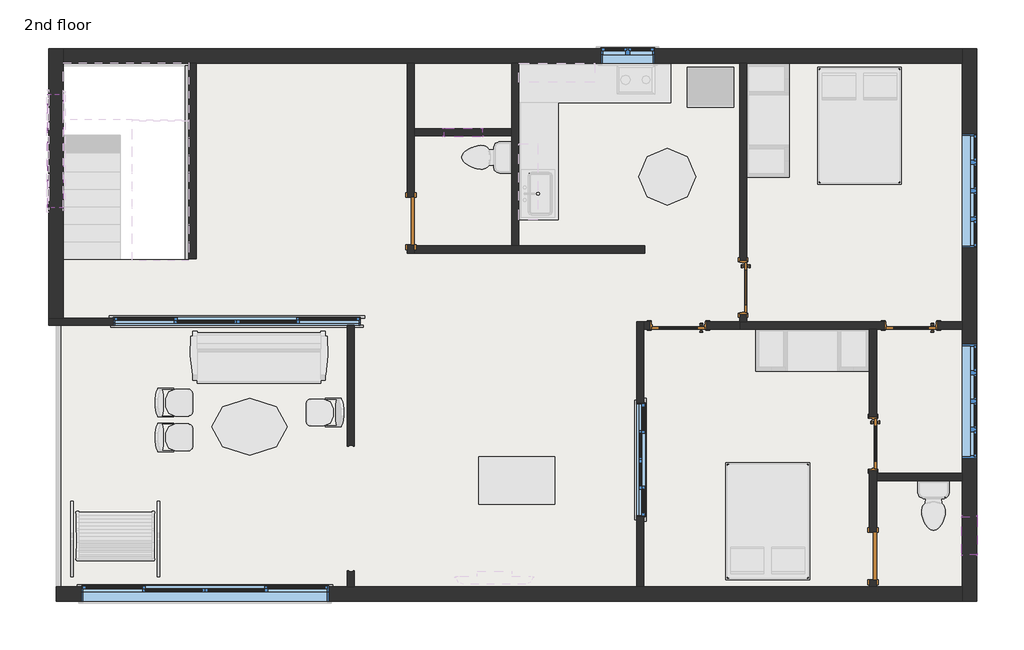
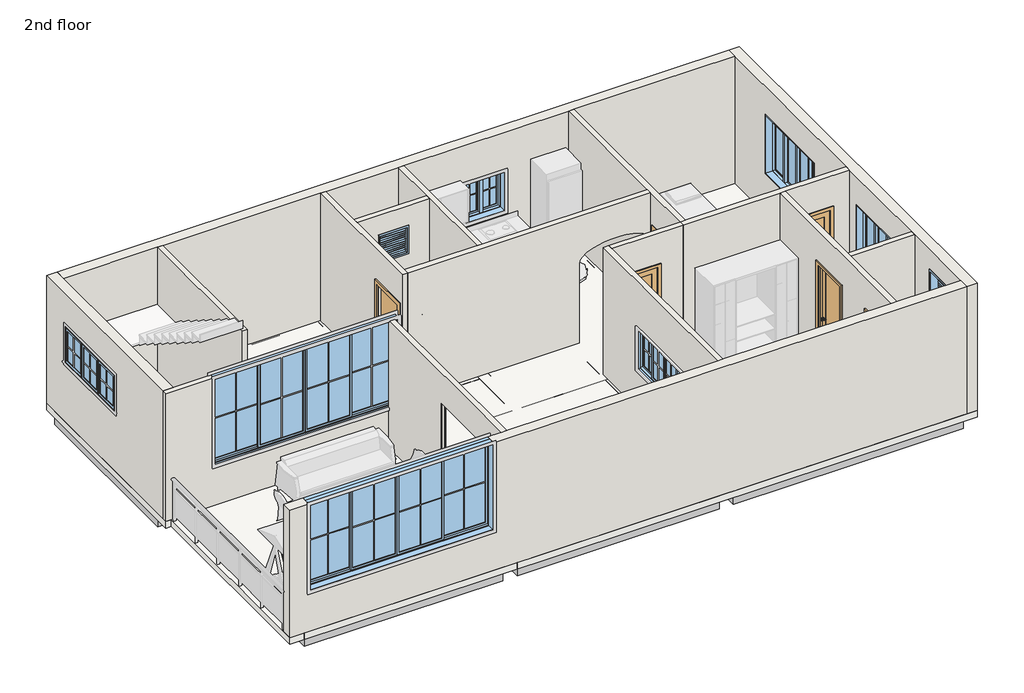
# One storey, part 1 of 2: 17 walls, 9 beams, 9 windows, 6 doors, 1 slab.
"""IFC4 building model written with IfcOpenShell, lengths in millimetres."""

from ifc_helpers import new_model, si_unit, point, frame, origin, place, context, project, spatial, polyline, ellipse_curve, trimmed, outline, extrude, faceted_brep, transform, mapped, element, save
from ifc_brep_helpers import plane_surface, extruded_surface, advanced_brep
from components import door_643e272e, door_51292941, door_214872d5, window_33d4544c, window_339605e1, window_5487fb6d, window_d39e7ecb, window_f2d8fef0, window_cbca41e3, window_8ea0b4a1, window_cd2bb1e7

model = new_model("IFC4")

# Units and contexts
model_context = context("Model", 3, world=origin())
ifc_project = project(units=[si_unit("LENGTHUNIT", "METRE", prefix="MILLI")], contexts=[model_context])

# Site, building, storey
site = spatial("IfcSite", under=ifc_project)
building = spatial("IfcBuilding", under=site)
storey = spatial("IfcBuildingStorey", under=building, Name="2nd floor", Elevation=7010.4)

# Beams
placement = place(None, origin())
element("IfcBeam", 1, ObjectType="Concrete-Rectangular Beam", at=placement, inside=storey, context=model_context, shape_type="Brep", body=[
    faceted_brep([(-12452.868339, 913.093496, 7010.4), (-12452.868339, 684.493496, 7010.4), (-8179.318339, 684.493496, 7010.4), (-8179.318339, 913.093496, 7010.4), (-12452.868339, 913.093496, 6705.6), (-8179.318339, 913.093496, 6705.6), (-12452.868339, 684.493496, 6705.6), (-8179.318339, 684.493496, 6705.6)], [[[0, 1, 2, 3]], [[4, 0, 3, 5]], [[6, 4, 5, 7]], [[1, 6, 7, 2]], [[1, 0, 4, 6]], [[3, 2, 7, 5]]]),
    faceted_brep([(1713.981661, 913.093496, 7010.4), (1713.981661, 684.493496, 7010.4), (1713.981661, 684.493496, 6705.6), (1713.981661, 913.093496, 6705.6), (-3226.216739, 684.493496, 7010.4), (-3226.216739, 913.093496, 7010.4), (-3226.216739, 913.093496, 6705.6), (-3226.216739, 684.493496, 6705.6), (469.381661, 913.093496, 7010.4), (240.781661, 913.093496, 7010.4), (-1613.418339, 913.093496, 7010.4), (-1842.018339, 913.093496, 7010.4), (469.381661, 913.093496, 6705.6), (240.781661, 913.093496, 6705.6), (-1613.418339, 913.093496, 6705.6), (-1842.018339, 913.093496, 6705.6)], [[[0, 1, 2, 3]], [[4, 5, 6, 7]], [[1, 0, 8, 9, 10, 11, 5, 4]], [[0, 3, 12, 13, 14, 15, 6, 5, 11, 10, 9, 8]], [[3, 2, 7, 6, 15, 14, 13, 12]], [[2, 1, 4, 7]]]),
    faceted_brep([(-7874.518339, 684.493496, 7010.4), (-7874.518339, 913.093496, 7010.4), (-7874.518339, 913.093496, 6705.6), (-7874.518339, 684.493496, 6705.6), (-3531.016739, 684.493496, 7010.4), (-3531.016739, 913.093496, 7010.4), (-5271.018339, 913.093496, 7010.4), (-5499.618339, 913.093496, 7010.4), (-6947.418339, 913.093496, 7010.4), (-7176.018339, 913.093496, 7010.4), (-3531.016739, 913.093496, 6705.6), (-5271.018339, 913.093496, 6705.6), (-5499.618339, 913.093496, 6705.6), (-6947.418339, 913.093496, 6705.6), (-7176.018339, 913.093496, 6705.6), (-3531.016739, 684.493496, 6705.6)], [[[0, 1, 2, 3]], [[1, 0, 4, 5, 6, 7, 8, 9]], [[2, 1, 9, 8, 7, 6, 5, 10, 11, 12, 13, 14]], [[3, 2, 14, 13, 12, 11, 10, 15]], [[0, 3, 15, 4]], [[5, 4, 15, 10]]]),
])
element("IfcBeam", 2, ObjectType="Concrete-Rectangular Beam", at=placement, inside=storey, context=model_context, shape_type="SweptSolid", body=[
    extrude(outline(polyline([(-12871.968339, 9244.293496), (-12643.368339, 9244.293496), (-12643.368339, 5415.243496), (-12871.968339, 5415.243496), (-12871.968339, 9244.293496)])), frame((0.0, 0.0, 6705.6), z_axis=(0.0, 0.0, 1.0), x_axis=(1.0, 0.0, 0.0)), (0.0, 0.0, 1.0), 304.8),
])
element("IfcBeam", 3, ObjectType="Concrete-Rectangular Beam", at=placement, inside=storey, context=model_context, shape_type="Brep", body=[
    faceted_brep([(-10452.618339, 5110.443496, 7010.4), (-10681.218339, 5110.443496, 7010.4), (-10681.218339, 5110.443496, 6705.6), (-10452.618339, 5110.443496, 6705.6), (-10452.618339, 5148.543496, 7010.4), (-10452.618339, 5377.143496, 7010.4), (-10452.618339, 9282.393496, 7010.4), (-10681.218339, 9282.393496, 7010.4), (-10681.218339, 5377.143496, 7010.4), (-10681.218339, 5148.543496, 7010.4), (-10681.218339, 9282.393496, 6705.6), (-10681.218339, 5377.143496, 6705.6), (-10681.218339, 5148.543496, 6705.6), (-10452.618339, 9282.393496, 6705.6), (-10452.618339, 5377.143496, 6705.6), (-10452.618339, 5148.543496, 6705.6)], [[[0, 1, 2, 3]], [[1, 0, 4, 5, 6, 7, 8, 9]], [[2, 1, 9, 8, 7, 10, 11, 12]], [[3, 2, 12, 11, 10, 13, 14, 15]], [[0, 3, 15, 14, 13, 6, 5, 4]], [[7, 6, 13, 10]]]),
])
element("IfcBeam", 4, ObjectType="Concrete-Rectangular Beam", at=placement, inside=storey, context=model_context, shape_type="Brep", body=[
    faceted_brep([(-10452.618339, 5377.143496, 7010.4), (-10452.618339, 5148.543496, 7010.4), (-8274.568339, 5148.543496, 7010.4), (-8274.568339, 5339.043496, 7010.4), (-7969.768339, 5339.043496, 7010.4), (-7969.768339, 5148.543496, 7010.4), (-7912.618339, 5148.543496, 7010.4), (-7912.618339, 5224.743496, 7010.4), (-7912.618339, 5377.143496, 7010.4), (-7912.618339, 5148.543496, 6705.6), (-7969.768339, 5148.543496, 6705.6), (-10452.618339, 5148.543496, 6705.6), (-10452.618339, 5377.143496, 6705.6), (-7912.618339, 5377.143496, 6705.6), (-7912.618339, 5224.743496, 6705.6), (-7969.768339, 5339.043496, 6705.6), (-8274.568339, 5339.043496, 6705.6), (-8274.568339, 5148.543496, 6705.6)], [[[0, 1, 2, 3, 4, 5, 6, 7, 8]], [[9, 6, 5, 10]], [[11, 12, 13, 14, 9, 10, 15, 16, 17]], [[12, 0, 8, 13]], [[1, 0, 12, 11]], [[8, 7, 6, 9, 14, 13]], [[16, 3, 2, 17]], [[3, 16, 15, 4]], [[4, 15, 10, 5]], [[1, 11, 17, 2]]]),
    faceted_brep([(-12643.368339, 5148.543496, 7010.4), (-12643.368339, 5377.143496, 7010.4), (-12643.368339, 5377.143496, 6705.6), (-12643.368339, 5148.543496, 6705.6), (-10681.218339, 5377.143496, 7010.4), (-10681.218339, 5148.543496, 7010.4), (-10681.218339, 5148.543496, 6705.6), (-10681.218339, 5377.143496, 6705.6)], [[[0, 1, 2, 3]], [[4, 5, 6, 7]], [[1, 0, 5, 4]], [[3, 2, 7, 6]], [[2, 1, 4, 7]], [[0, 3, 6, 5]]]),
])
element("IfcBeam", 5, ObjectType="Concrete-Rectangular Beam", at=placement, inside=storey, context=model_context, shape_type="Brep", body=[
    faceted_brep([(-7912.618339, 5148.543496, 7010.4), (-7969.768339, 5148.543496, 7010.4), (-7969.768339, 5110.443496, 7010.4), (-8141.218339, 5110.443496, 7010.4), (-8141.218339, 913.093496, 7010.4), (-7912.618339, 913.093496, 7010.4), (-7912.618339, 4996.143496, 7010.4), (-7912.618339, 5148.543496, 6705.6), (-7912.618339, 913.093496, 6705.6), (-7912.618339, 4996.143496, 6705.6), (-7969.768339, 5148.543496, 6705.6), (-8141.218339, 913.093496, 6705.6), (-8141.218339, 5110.443496, 6705.6), (-7969.768339, 5110.443496, 6705.6)], [[[0, 1, 2, 3, 4, 5, 6]], [[7, 0, 6, 5, 8, 9]], [[10, 7, 9, 8, 11, 12, 13]], [[3, 12, 11, 4]], [[0, 7, 10, 1]], [[2, 13, 12, 3]], [[13, 2, 1, 10]], [[5, 4, 11, 8]]]),
])
element("IfcBeam", 6, ObjectType="Concrete-Rectangular Beam", at=placement, inside=storey, context=model_context, shape_type="Brep", body=[
    faceted_brep([(-6947.418339, 9282.393496, 7010.4), (-7176.018339, 9282.393496, 7010.4), (-7176.018339, 5224.743496, 7010.4), (-7176.018339, 4996.143496, 7010.4), (-7176.018339, 913.093496, 7010.4), (-6947.418339, 913.093496, 7010.4), (-6947.418339, 4996.143496, 7010.4), (-6947.418339, 5224.743496, 7010.4), (-6947.418339, 6213.330971, 7010.4), (-6947.418339, 6441.9657932, 7010.4), (-6947.418339, 8094.943496, 7010.4), (-6947.418339, 8323.543496, 7010.4), (-7176.018339, 9282.393496, 6705.6), (-7176.018339, 5224.743496, 6705.6), (-7176.018339, 4996.143496, 6705.6), (-7176.018339, 913.093496, 6705.6), (-6947.418339, 9282.393496, 6705.6), (-6947.418339, 8323.543496, 6705.6), (-6947.418339, 8094.943496, 6705.6), (-6947.418339, 6441.9657932, 6705.6), (-6947.418339, 6213.330971, 6705.6), (-6947.418339, 5224.743496, 6705.6), (-6947.418339, 4996.143496, 6705.6), (-6947.418339, 913.093496, 6705.6)], [[[0, 1, 2, 3, 4, 5, 6, 7, 8, 9, 10, 11]], [[1, 12, 13, 14, 15, 4, 3, 2]], [[12, 16, 17, 18, 19, 20, 21, 22, 23, 15, 14, 13]], [[16, 0, 11, 10, 9, 8, 7, 6, 5, 23, 22, 21, 20, 19, 18, 17]], [[1, 0, 16, 12]], [[5, 4, 15, 23]]]),
])
element("IfcBeam", 7, ObjectType="Concrete-Rectangular Beam", at=placement, inside=storey, context=model_context, shape_type="Brep", body=[
    faceted_brep([(-5271.018339, 9282.393496, 7010.4), (-5499.618339, 9282.393496, 7010.4), (-5499.618339, 8323.543496, 7010.4), (-5499.618339, 8094.943496, 7010.4), (-5499.618339, 6416.6943502, 7010.4), (-5499.618339, 6188.059528, 7010.4), (-5499.618339, 5224.743496, 7010.4), (-5499.618339, 4996.143496, 7010.4), (-5499.618339, 913.093496, 7010.4), (-5271.018339, 913.093496, 7010.4), (-5271.018339, 4996.143496, 7010.4), (-5271.018339, 5224.743496, 7010.4), (-5271.018339, 6184.0693001, 7010.4), (-5271.018339, 6412.7041223, 7010.4), (-5499.618339, 9282.393496, 6705.6), (-5499.618339, 8323.543496, 6705.6), (-5499.618339, 8094.943496, 6705.6), (-5499.618339, 6416.6943502, 6705.6), (-5499.618339, 6188.059528, 6705.6), (-5499.618339, 5224.743496, 6705.6), (-5499.618339, 4996.143496, 6705.6), (-5499.618339, 913.093496, 6705.6), (-5271.018339, 9282.393496, 6705.6), (-5271.018339, 6412.7041223, 6705.6), (-5271.018339, 6184.0693001, 6705.6), (-5271.018339, 5224.743496, 6705.6), (-5271.018339, 4996.143496, 6705.6), (-5271.018339, 913.093496, 6705.6)], [[[0, 1, 2, 3, 4, 5, 6, 7, 8, 9, 10, 11, 12, 13]], [[1, 14, 15, 16, 17, 18, 19, 20, 21, 8, 7, 6, 5, 4, 3, 2]], [[14, 22, 23, 24, 25, 26, 27, 21, 20, 19, 18, 17, 16, 15]], [[22, 0, 13, 12, 11, 10, 9, 27, 26, 25, 24, 23]], [[1, 0, 22, 14]], [[9, 8, 21, 27]]]),
])
element("IfcBeam", 8, ObjectType="Concrete-Rectangular Beam", at=placement, inside=storey, context=model_context, shape_type="Brep", body=[
    faceted_brep([(-7176.018339, 4996.143496, 7010.4), (-7176.018339, 5224.743496, 7010.4), (-7912.618339, 5224.743496, 7010.4), (-7912.618339, 5148.543496, 7010.4), (-7912.618339, 4996.143496, 7010.4), (-7176.018339, 5224.743496, 6705.6), (-7912.618339, 5224.743496, 6705.6), (-7176.018339, 4996.143496, 6705.6), (-7912.618339, 4996.143496, 6705.6), (-7912.618339, 5148.543496, 6705.6)], [[[0, 1, 2, 3, 4]], [[1, 5, 6, 2]], [[5, 7, 8, 9, 6]], [[4, 8, 7, 0]], [[1, 0, 7, 5]], [[8, 4, 3, 2, 6, 9]]]),
    faceted_brep([(-6947.418339, 4996.143496, 7010.4), (-6947.418339, 5224.743496, 7010.4), (-6947.418339, 5224.743496, 6705.6), (-6947.418339, 4996.143496, 6705.6), (-5499.618339, 4996.143496, 7010.4), (-5499.618339, 5224.743496, 7010.4), (-5499.618339, 5224.743496, 6705.6), (-5499.618339, 4996.143496, 6705.6)], [[[0, 1, 2, 3]], [[1, 0, 4, 5]], [[2, 1, 5, 6]], [[3, 2, 6, 7]], [[0, 3, 7, 4]], [[5, 4, 7, 6]]]),
    faceted_brep([(-5271.018339, 4996.143496, 7010.4), (-5271.018339, 5224.743496, 7010.4), (-5271.018339, 5224.743496, 6705.6), (-5271.018339, 4996.143496, 6705.6), (-3492.916739, 4996.143496, 7010.4), (-3264.316739, 4996.143496, 7010.4), (-1842.018339, 4996.143496, 7010.4), (-1842.018339, 5053.293496, 7010.4), (-2089.668339, 5053.293496, 7010.4), (-2089.668339, 5224.743496, 7010.4), (-3264.316739, 5224.743496, 7010.4), (-3492.916739, 5224.743496, 7010.4), (-2089.668339, 5224.743496, 6705.6), (-3264.316739, 5224.743496, 6705.6), (-3492.916739, 5224.743496, 6705.6), (-2089.668339, 5053.293496, 6705.6), (-1842.018339, 5053.293496, 6705.6), (-1842.018339, 4996.143496, 6705.6), (-3264.316739, 4996.143496, 6705.6), (-3492.916739, 4996.143496, 6705.6)], [[[0, 1, 2, 3]], [[1, 0, 4, 5, 6, 7, 8, 9, 10, 11]], [[2, 1, 11, 10, 9, 12, 13, 14]], [[3, 2, 14, 13, 12, 15, 16, 17, 18, 19]], [[0, 3, 19, 18, 17, 6, 5, 4]], [[6, 17, 16, 7]], [[15, 8, 7, 16]], [[8, 15, 12, 9]]]),
    faceted_brep([(-1613.418339, 4996.143496, 7010.4), (-1613.418339, 5224.743496, 7010.4), (-1613.418339, 5224.743496, 6705.6), (-1613.418339, 4996.143496, 6705.6), (240.781661, 4996.143496, 7010.4), (469.381661, 4996.143496, 7010.4), (1790.181661, 4996.143496, 7010.4), (1790.181661, 5224.743496, 7010.4), (1790.181661, 5224.743496, 6705.6), (1790.181661, 4996.143496, 6705.6), (469.381661, 4996.143496, 6705.6), (240.781661, 4996.143496, 6705.6)], [[[0, 1, 2, 3]], [[1, 0, 4, 5, 6, 7]], [[3, 2, 8, 9, 10, 11]], [[0, 3, 11, 10, 9, 6, 5, 4]], [[2, 1, 7, 8]], [[7, 6, 9, 8]]]),
])
element("IfcBeam", 9, ObjectType="Concrete-Rectangular Beam", at=placement, inside=storey, context=model_context, shape_type="SweptSolid", body=[
    extrude(outline(polyline([(-3492.916739, 9282.393496), (-3264.316739, 9282.393496), (-3264.316739, 6377.6770156), (-3492.916739, 6381.6672435), (-3492.916739, 9282.393496)])), frame((0.0, 0.0, 6705.6), z_axis=(0.0, 0.0, 1.0), x_axis=(1.0, 0.0, 0.0)), (0.0, 0.0, 1.0), 304.8),
    extrude(outline(polyline([(-3492.916739, 6153.0324213), (-3264.316739, 6149.0421934), (-3264.316739, 5224.743496), (-3492.916739, 5224.743496), (-3492.916739, 6153.0324213)])), frame((0.0, 0.0, 6705.6), z_axis=(0.0, 0.0, 1.0), x_axis=(1.0, 0.0, 0.0)), (0.0, 0.0, 1.0), 304.8),
    extrude(outline(polyline([(-3492.916739, 4996.143496), (-3264.316739, 4996.143496), (-3264.316739, 913.093496), (-3492.916739, 913.093496), (-3492.916739, 4996.143496)])), frame((0.0, 0.0, 6705.6), z_axis=(0.0, 0.0, 1.0), x_axis=(1.0, 0.0, 0.0)), (0.0, 0.0, 1.0), 304.8),
])

# Doors
door_shape = door_643e272e(model_context)
element("IfcDoor", 10, ObjectType="Door-Interior-Single-1_Panel-Wood : 32\" x 84\"", at=placement, inside=storey, context=model_context, shape_type="MappedRepresentation", body=[
    mapped(door_shape, transform((-1724.543339, 5720.043496, 7010.4), x_axis=(0.0, -1.0, 0.0), y_axis=(1.0, 0.0, 0.0), z_axis=(0.0, 0.0, 1.0))),
])
element("IfcDoor", 11, ObjectType="Door-Interior-Single-1_Panel-Wood : 32\" x 84\"", at=placement, inside=storey, context=model_context, shape_type="MappedRepresentation", body=[
    mapped(door_shape, transform((358.256661, 3211.793496, 7010.4), x_axis=(0.0, -1.0, 0.0), y_axis=(1.0, 0.0, 0.0), z_axis=(0.0, 0.0, 1.0))),
])
element("IfcDoor", 12, ObjectType="Door-Interior-Single-1_Panel-Wood : 32\" x 84\"", at=placement, inside=storey, context=model_context, shape_type="MappedRepresentation", body=[
    mapped(door_shape, transform((964.681661, 5107.268496, 7010.4), x_axis=(-1.0, 0.0, 0.0), y_axis=(0.0, -1.0, 0.0), z_axis=(0.0, 0.0, 1.0))),
])
door_2_shape = door_51292941(model_context)
element("IfcDoor", 13, ObjectType="Door-Interior-Single-1_Panel-Wood : 34\" x 84\"", at=placement, inside=storey, context=model_context, shape_type="MappedRepresentation", body=[
    mapped(door_2_shape, transform((-2769.016739, 5107.268496, 7010.4), x_axis=(-1.0, 0.0, 0.0), y_axis=(0.0, -1.0, 0.0), z_axis=(0.0, 0.0, 1.0))),
])
door_3_shape = door_214872d5(model_context)
element("IfcDoor", 14, ObjectType="Single-Flush : 30\" x 84\"", at=placement, inside=storey, context=model_context, shape_type="MappedRepresentation", body=[
    mapped(door_3_shape, transform((355.081661, 1408.393496, 7010.4), x_axis=(0.0, -1.0, 0.0), y_axis=(1.0, 0.0, 0.0), z_axis=(0.0, 0.0, 1.0))),
])
element("IfcDoor", 15, ObjectType="Single-Flush : 30\" x 84\"", at=placement, inside=storey, context=model_context, shape_type="MappedRepresentation", body=[
    mapped(door_3_shape, transform((-7061.718339, 6786.843496, 7010.4), x_axis=(0.0, -1.0, 0.0), y_axis=(1.0, 0.0, 0.0), z_axis=(0.0, 0.0, 1.0))),
])

# Slab
element("IfcSlab", 16, ObjectType="Generic - 6\"", at=placement, inside=storey, context=model_context, shape_type="SweptSolid", body=[
    extrude(outline(polyline([(2018.781661, 9549.093496), (2018.781661, 684.493496), (-12757.668339, 684.493496), (-12757.668339, 5110.443496), (-12871.968339, 5110.443496), (-12871.968339, 9549.093496), (2018.781661, 9549.093496)]), holes=[polyline([(-10624.068339, 9320.493496), (-12643.368339, 9320.493496), (-12643.368339, 6177.243496), (-10624.068339, 6177.243496), (-10624.068339, 9320.493496)])]), frame((0.0, 0.0, 6858.0), z_axis=(0.0, 0.0, 1.0), x_axis=(1.0, 0.0, 0.0)), (0.0, 0.0, 1.0), 152.4),
])

# Walls
element("IfcWall", 17, ObjectType="Generic - 4.5\"", at=placement, inside=storey, context=model_context, shape_type="SweptSolid", body=[
    extrude(outline(polyline([(-10624.068339, 6177.243496), (-10624.068339, 9320.493496), (-10509.768339, 9320.493496), (-10509.768339, 6177.243496), (-10624.068339, 6177.243496)])), frame((0.0, 0.0, 7010.4), z_axis=(0.0, 0.0, 1.0), x_axis=(1.0, 0.0, 0.0)), (0.0, 0.0, 1.0), 2895.6),
])
element("IfcWall", 18, ObjectType="Generic - 4.5\"", at=placement, inside=storey, context=model_context, shape_type="Brep", body=[
    faceted_brep([(-7118.868339, 6405.843496, 9144.0), (-7118.868339, 6405.843496, 7010.4), (-7118.868339, 6272.493496, 7010.4), (-7118.868339, 6272.493496, 9906.0), (-7118.868339, 9320.493496, 9906.0), (-7118.868339, 9320.493496, 7010.4), (-7118.868339, 7167.843496, 7010.4), (-7118.868339, 7167.843496, 9144.0), (-7004.568339, 6272.493496, 7010.4), (-7004.568339, 6386.793496, 7010.4), (-7004.568339, 6405.843496, 7010.4), (-7004.568339, 6405.843496, 9144.0), (-7004.568339, 7167.843496, 9144.0), (-7004.568339, 7167.843496, 7010.4), (-7004.568339, 8152.093496, 7010.4), (-7004.568339, 8266.393496, 7010.4), (-7004.568339, 9320.493496, 7010.4), (-7004.568339, 9320.493496, 9906.0), (-7004.568339, 8266.393496, 9906.0), (-7004.568339, 8152.093496, 9906.0), (-7004.568339, 6386.793496, 9906.0), (-7004.568339, 6272.493496, 9906.0)], [[[0, 1, 2, 3, 4, 5, 6, 7]], [[8, 9, 10, 11, 12, 13, 14, 15, 16, 17, 18, 19, 20, 21]], [[6, 5, 16, 15, 14, 13]], [[2, 1, 10, 9, 8]], [[4, 3, 21, 20, 19, 18, 17]], [[3, 2, 8, 21]], [[5, 4, 17, 16]], [[11, 10, 1, 0]], [[12, 11, 0, 7]], [[13, 12, 7, 6]]]),
])
element("IfcWall", 19, ObjectType="Generic - 4.5\"", at=placement, inside=storey, context=model_context, shape_type="Brep", body=[
    faceted_brep([(-5442.468339, 9320.493496, 7010.4), (-5442.468339, 8266.393496, 7010.4), (-5442.468339, 8152.093496, 7010.4), (-5442.468339, 6386.793496, 7010.4), (-5442.468339, 6386.793496, 9906.0), (-5442.468339, 8152.093496, 9906.0), (-5442.468339, 8266.393496, 9906.0), (-5442.468339, 9320.493496, 9906.0), (-5328.168339, 9320.493496, 7010.4), (-5328.168339, 9320.493496, 9906.0), (-5328.168339, 6386.793496, 9906.0), (-5328.168339, 6386.793496, 7010.4)], [[[0, 1, 2, 3, 4, 5, 6, 7]], [[8, 9, 10, 11]], [[3, 2, 1, 0, 8, 11]], [[7, 6, 5, 4, 10, 9]], [[4, 3, 11, 10]], [[0, 7, 9, 8]]]),
])
element("IfcWall", 20, ObjectType="Generic - 4.5\"", at=placement, inside=storey, context=model_context, shape_type="Brep", body=[
    faceted_brep([(-1784.868339, 5167.593496, 9906.0), (-1784.868339, 6272.493496, 9906.0), (-1784.868339, 6386.793496, 9906.0), (-1784.868339, 9320.493496, 9906.0), (-1784.868339, 9320.493496, 7010.4), (-1784.868339, 6386.793496, 7010.4), (-1784.868339, 6272.493496, 7010.4), (-1784.868339, 6151.843496, 7010.4), (-1784.868339, 6151.843496, 9169.4), (-1784.868339, 5288.243496, 9169.4), (-1784.868339, 5288.243496, 7010.4), (-1784.868339, 5167.593496, 7010.4), (-1670.568339, 9320.493496, 9906.0), (-1670.568339, 5167.593496, 9906.0), (-1670.568339, 5167.593496, 7010.4), (-1670.568339, 5288.243496, 7010.4), (-1670.568339, 5288.243496, 9169.4), (-1670.568339, 6151.843496, 9169.4), (-1670.568339, 6151.843496, 7010.4), (-1670.568339, 9320.493496, 7010.4)], [[[0, 1, 2, 3, 4, 5, 6, 7, 8, 9, 10, 11]], [[12, 13, 14, 15, 16, 17, 18, 19]], [[14, 11, 10, 15]], [[4, 19, 18, 7, 6, 5]], [[3, 2, 1, 0, 13, 12]], [[0, 11, 14, 13]], [[4, 3, 12, 19]], [[9, 16, 15, 10]], [[16, 9, 8, 17]], [[17, 8, 7, 18]]]),
])
element("IfcWall", 21, ObjectType="Generic - 4.5\"", at=placement, inside=storey, context=model_context, shape_type="Brep", body=[
    faceted_brep([(-1784.868339, 5167.593496, 9906.0), (-1670.568339, 5167.593496, 9906.0), (1790.181661, 5167.593496, 9906.0), (1790.181661, 5167.593496, 7010.4), (1396.481661, 5167.593496, 7010.4), (1396.481661, 5167.593496, 9169.4), (532.881661, 5167.593496, 9169.4), (532.881661, 5167.593496, 7010.4), (-1670.568339, 5167.593496, 7010.4), (-1784.868339, 5167.593496, 7010.4), (1790.181661, 5053.293496, 9906.0), (412.231661, 5053.293496, 9906.0), (297.931661, 5053.293496, 9906.0), (-1784.868339, 5053.293496, 9906.0), (-1784.868339, 5053.293496, 7010.4), (297.931661, 5053.293496, 7010.4), (412.231661, 5053.293496, 7010.4), (532.881661, 5053.293496, 7010.4), (532.881661, 5053.293496, 9169.4), (1396.481661, 5053.293496, 9169.4), (1396.481661, 5053.293496, 7010.4), (1790.181661, 5053.293496, 7010.4)], [[[0, 1, 2, 3, 4, 5, 6, 7, 8, 9]], [[10, 11, 12, 13, 14, 15, 16, 17, 18, 19, 20, 21]], [[3, 21, 20, 4]], [[14, 9, 8, 7, 17, 16, 15]], [[2, 1, 0, 13, 12, 11, 10]], [[3, 2, 10, 21]], [[0, 9, 14, 13]], [[6, 18, 17, 7]], [[18, 6, 5, 19]], [[19, 5, 4, 20]]]),
])
element("IfcWall", 22, ObjectType="Generic - 4.5\"", at=placement, inside=storey, context=model_context, shape_type="AdvancedBrep", body=[
    advanced_brep(
    [(-1784.868339, 6272.493496, 9906.0), (-7004.568339, 6272.493496, 9906.0), (-7004.568339, 6272.493496, 7010.4), (-3308.868339, 6272.493496, 7010.4), (-3308.868339, 6272.493496, 8839.2), (-1784.868339, 6272.493496, 8839.2), (-7004.568339, 6386.793496, 9906.0), (-5442.468339, 6386.793496, 9906.0), (-5328.168339, 6386.793496, 9906.0), (-1784.868339, 6386.793496, 9906.0), (-1784.868339, 6386.793496, 8839.2), (-3308.868339, 6386.793496, 8839.2), (-3308.868339, 6386.793496, 7010.4), (-5328.168339, 6386.793496, 7010.4), (-5442.468339, 6386.793496, 7010.4), (-7004.568339, 6386.793496, 7010.4)],
    [
        (0, 1),
        (1, 2),
        (2, 3),
        (3, 4),
        (4, 5, ellipse_curve(frame((-2546.868339, 6272.493496, 8839.2), z_axis=(0.0, 1.0, 0.0), x_axis=(1.0, 0.0, 0.0)), 762.0, 304.8)),
        (5, 0),
        (6, 7),
        (7, 8),
        (8, 9),
        (9, 10),
        (10, 11, ellipse_curve(frame((-2546.868339, 6386.793496, 8839.2), z_axis=(0.0, -1.0, 0.0), x_axis=(1.0, 0.0, 0.0)), 762.0, 304.8)),
        (11, 12),
        (12, 13),
        (13, 14),
        (14, 15),
        (15, 6),
        (2, 15),
        (12, 3),
        (0, 9),
        (6, 1),
        (5, 10),
        (4, 11),
    ],
    [
        plane_surface(frame((-7061.718339, 6272.493496, 7010.4), z_axis=(0.0, -1.0, 0.0), x_axis=(1.0, 0.0, 0.0))),
        plane_surface(frame((-7061.718339, 6386.793496, 7010.4), z_axis=(0.0, 1.0, 0.0), x_axis=(-1.0, 0.0, 0.0))),
        plane_surface(frame((-7061.718339, 6272.493496, 7010.4), z_axis=(0.0, 0.0, -1.0), x_axis=(0.0, 1.0, 0.0))),
        plane_surface(frame((-1727.718339, 6272.493496, 9906.0), z_axis=(0.0, 0.0, 1.0), x_axis=(0.0, 1.0, 0.0))),
        plane_surface(frame((-7004.568339, 9377.643496, 7010.4), z_axis=(-1.0, 0.0, 0.0), x_axis=(0.0, 1.0, 0.0))),
        plane_surface(frame((-1784.868339, 9377.643496, 7010.4), z_axis=(1.0, 0.0, 0.0), x_axis=(0.0, -1.0, 0.0))),
        extruded_surface(trimmed(ellipse_curve(frame((-2546.868339, 7796.493496, 8839.2), z_axis=(0.0, -1.0, 0.0), x_axis=(1.0, 0.0, 0.0)), 762.0, 304.8), [point((-1784.868339, 7796.493496, 8839.2))], [point((-3308.868339, 7796.493496, 8839.2))], True, "CARTESIAN"), (0.0, 3047.999999999999, 0.0), 3047.999999999999),
        plane_surface(frame((-3308.868339, 4748.493496, 8839.2), z_axis=(1.0, 0.0, 0.0), x_axis=(0.0, 1.0, 0.0))),
    ],
    [
        (0, [[1, 2, 3, 4, 5, 6]]),
        (1, [[7, 8, 9, 10, 11, 12, 13, 14, 15, 16]]),
        (2, [[17, -15, -14, -13, 18, -3]]),
        (3, [[-1, 19, -9, -8, -7, 20]]),
        (4, [[-2, -20, -16, -17]]),
        (5, [[-19, -6, 21, -10]]),
        (6, [[22, -11, -21, -5]]),
        (7, [[-22, -4, -18, -12]]),
    ],
),
])
element("IfcWall", 23, ObjectType="Generic - 4.5\"", at=placement, inside=storey, context=model_context, shape_type="Brep", body=[
    faceted_brep([(297.931661, 913.093496, 9906.0), (297.931661, 5053.293496, 9906.0), (297.931661, 5053.293496, 7010.4), (297.931661, 3643.593496, 7010.4), (297.931661, 3643.593496, 9169.4), (297.931661, 2779.993496, 9169.4), (297.931661, 2779.993496, 7010.4), (297.931661, 1789.393496, 7010.4), (297.931661, 1789.393496, 9144.0), (297.931661, 1027.393496, 9144.0), (297.931661, 1027.393496, 7010.4), (297.931661, 913.093496, 7010.4), (412.231661, 5053.293496, 9906.0), (412.231661, 2735.543496, 9906.0), (412.231661, 2621.243496, 9906.0), (412.231661, 913.093496, 9906.0), (412.231661, 913.093496, 7010.4), (412.231661, 1027.393496, 7010.4), (412.231661, 1027.393496, 9144.0), (412.231661, 1789.393496, 9144.0), (412.231661, 1789.393496, 7010.4), (412.231661, 2621.243496, 7010.4), (412.231661, 2735.543496, 7010.4), (412.231661, 2779.993496, 7010.4), (412.231661, 2779.993496, 9169.4), (412.231661, 3643.593496, 9169.4), (412.231661, 3643.593496, 7010.4), (412.231661, 5053.293496, 7010.4)], [[[0, 1, 2, 3, 4, 5, 6, 7, 8, 9, 10, 11]], [[12, 13, 14, 15, 16, 17, 18, 19, 20, 21, 22, 23, 24, 25, 26, 27]], [[2, 27, 26, 3]], [[16, 11, 10, 17]], [[20, 7, 6, 23, 22, 21]], [[1, 0, 15, 14, 13, 12]], [[2, 1, 12, 27]], [[0, 11, 16, 15]], [[18, 17, 10, 9]], [[19, 18, 9, 8]], [[20, 19, 8, 7]], [[5, 24, 23, 6]], [[24, 5, 4, 25]], [[25, 4, 3, 26]]]),
])
element("IfcWall", 24, ObjectType="Generic - 4.5\"", at=placement, inside=storey, context=model_context, shape_type="SweptSolid", body=[
    extrude(outline(polyline([(1790.181661, 2621.243496), (412.231661, 2621.243496), (412.231661, 2735.543496), (1790.181661, 2735.543496), (1790.181661, 2621.243496)])), frame((0.0, 0.0, 7010.4), z_axis=(0.0, 0.0, 1.0), x_axis=(1.0, 0.0, 0.0)), (0.0, 0.0, 1.0), 2895.6),
])
element("IfcWall", 25, ObjectType="Generic - 4.5\"", at=placement, inside=storey, context=model_context, shape_type="Brep", body=[
    faceted_brep([(-3435.766739, 5167.593496, 7010.4), (-3435.766739, 913.093496, 7010.4), (-3435.766739, 913.093496, 9906.0), (-3435.766739, 5167.593496, 9906.0), (-3435.766739, 2040.218496, 8839.2), (-3435.766739, 2040.218496, 7924.8), (-3435.766739, 3869.018496, 7924.8), (-3435.766739, 3869.018496, 8839.2), (-3321.466739, 5167.593496, 7010.4), (-3321.466739, 5167.593496, 9906.0), (-3321.466739, 5053.293496, 9906.0), (-3321.466739, 913.093496, 9906.0), (-3321.466739, 913.093496, 7010.4), (-3321.466739, 5053.293496, 7010.4), (-3321.466739, 2040.218496, 8839.2), (-3321.466739, 3869.018496, 8839.2), (-3321.466739, 3869.018496, 7924.8), (-3321.466739, 2040.218496, 7924.8)], [[[0, 1, 2, 3], [4, 5, 6, 7]], [[8, 9, 10, 11, 12, 13], [14, 15, 16, 17]], [[1, 0, 8, 13, 12]], [[3, 2, 11, 10, 9]], [[2, 1, 12, 11]], [[0, 3, 9, 8]], [[5, 4, 14, 17]], [[6, 5, 17, 16]], [[7, 6, 16, 15]], [[4, 7, 15, 14]]]),
])
element("IfcWall", 26, ObjectType="Generic - 4.5\"", at=placement, inside=storey, context=model_context, shape_type="Brep", body=[
    faceted_brep([(-8084.068339, 913.093496, 7010.4), (-8084.068339, 913.093496, 9906.0), (-8084.068339, 5110.443496, 9906.0), (-8084.068339, 5110.443496, 7924.8), (-8084.068339, 5224.743496, 7924.8), (-8084.068339, 5224.743496, 7010.4), (-8084.068339, 5110.443496, 7010.4), (-8084.068339, 3170.393496, 7010.4), (-8084.068339, 3170.393496, 9219.4), (-8084.068339, 1170.393496, 9219.4), (-8084.068339, 1170.393496, 7010.4), (-7969.768339, 913.093496, 9906.0), (-7969.768339, 913.093496, 7010.4), (-7969.768339, 1170.393496, 7010.4), (-7969.768339, 1170.393496, 9219.4), (-7969.768339, 3170.393496, 9219.4), (-7969.768339, 3170.393496, 7010.4), (-7969.768339, 5224.743496, 7010.4), (-7969.768339, 5224.743496, 7924.8), (-7969.768339, 5110.443496, 7924.8), (-7969.768339, 5110.443496, 9906.0), (-8059.7683389, 1170.393496, 7010.4), (-8059.7683389, 1155.393496, 7010.4), (-7989.7683389, 1155.393496, 7010.4), (-7989.7683389, 1170.393496, 7010.4), (-7989.7683389, 3170.393496, 7010.4), (-7989.7683389, 3185.393496, 7010.4), (-8059.7683389, 3185.393496, 7010.4), (-8059.7683389, 3170.393496, 7010.4), (-7989.7683389, 1170.393496, 9219.4), (-7989.7683389, 3170.393496, 9219.4), (-8059.7683389, 3170.393496, 9219.4), (-8059.7683389, 1170.393496, 9219.4), (-8059.7683389, 3185.393496, 9234.4), (-8059.7683389, 1155.393496, 9234.4), (-7989.7683389, 1155.393496, 9234.4), (-7989.7683389, 3185.393496, 9234.4)], [[[0, 1, 2, 3, 4, 5, 6, 7, 8, 9, 10]], [[11, 12, 13, 14, 15, 16, 17, 18, 19, 20]], [[12, 0, 10, 21, 22, 23, 24, 13]], [[5, 17, 16, 25, 26, 27, 28, 7, 6]], [[1, 11, 20, 2]], [[1, 0, 12, 11]], [[17, 5, 4, 18]], [[29, 30, 15, 14]], [[31, 32, 9, 8]], [[28, 31, 8, 7]], [[32, 21, 10, 9]], [[32, 31, 28, 27, 33, 34, 22, 21]], [[22, 34, 35, 23]], [[30, 29, 24, 23, 35, 36, 26, 25]], [[24, 29, 14, 13]], [[30, 25, 16, 15]], [[33, 27, 26, 36]], [[34, 33, 36, 35]], [[19, 3, 2, 20]], [[3, 19, 18, 4]]]),
])
element("IfcWall", 27, ObjectType="Generic - 4.5\"", at=placement, inside=storey, context=model_context, shape_type="Brep", body=[
    faceted_brep([(-8084.068339, 5224.743496, 7010.4), (-12643.368339, 5224.743496, 7010.4), (-12871.968339, 5224.743496, 7010.4), (-12871.968339, 5224.743496, 9906.0), (-12643.368339, 5224.743496, 9906.0), (-11836.918339, 5224.743496, 9906.0), (-11836.918339, 5224.743496, 7924.8), (-8084.068339, 5224.743496, 7924.8), (-12871.968339, 5110.443496, 7010.4), (-8084.068339, 5110.443496, 7010.4), (-8084.068339, 5110.443496, 7924.8), (-11836.918339, 5110.443496, 7924.8), (-11836.918339, 5110.443496, 9906.0), (-12871.968339, 5110.443496, 9906.0)], [[[0, 1, 2, 3, 4, 5, 6, 7]], [[8, 9, 10, 11, 12, 13]], [[2, 1, 0, 9, 8]], [[3, 13, 12, 5, 4]], [[9, 0, 7, 10]], [[3, 2, 8, 13]], [[6, 11, 10, 7]], [[11, 6, 5, 12]]]),
])
element("IfcWall", 28, ObjectType="Generic - 4.5\"", at=placement, inside=storey, context=model_context, shape_type="SweptSolid", body=[
    extrude(outline(polyline([(9906.0, -1784.868339), (9906.0, -3321.466739), (7010.4, -3321.466739), (7010.4, -3226.216739), (9169.4, -3226.216739), (9169.4, -2311.816739), (7010.4, -2311.816739), (7010.4, -1784.868339), (9906.0, -1784.868339)])), frame((0.0, 5053.293496, 0.0), z_axis=(0.0, 1.0, 0.0), x_axis=(0.0, 0.0, 1.0)), (0.0, 0.0, 1.0), 114.3),
])
element("IfcWall", 29, ObjectType="Generic - 4.5\"", at=placement, inside=storey, context=model_context, shape_type="SweptSolid", body=[
    extrude(outline(polyline([(7010.4, -7004.568339), (7010.4, -5442.468339), (9906.0, -5442.468339), (9906.0, -7004.568339), (7010.4, -7004.568339)]), holes=[polyline([(9448.8, -6528.318339), (9448.8, -5918.718339), (8839.2, -5918.718339), (8839.2, -6528.318339), (9448.8, -6528.318339)])]), frame((0.0, 8152.093496, 0.0), z_axis=(0.0, 1.0, 0.0), x_axis=(0.0, 0.0, 1.0)), (0.0, 0.0, 1.0), 114.3),
])
element("IfcWall", 30, ObjectType="Generic - 9\"", at=placement, inside=storey, context=model_context, shape_type="Brep", body=[
    faceted_brep([(1790.181661, 9549.093496, 7010.4), (1790.181661, 9320.493496, 7010.4), (1790.181661, 5167.593496, 7010.4), (1790.181661, 5053.293496, 7010.4), (1790.181661, 2735.543496, 7010.4), (1790.181661, 2621.243496, 7010.4), (1790.181661, 913.093496, 7010.4), (1790.181661, 684.493496, 7010.4), (1790.181661, 684.493496, 9906.0), (1790.181661, 913.093496, 9906.0), (1790.181661, 2621.243496, 9906.0), (1790.181661, 2735.543496, 9906.0), (1790.181661, 5053.293496, 9906.0), (1790.181661, 5167.593496, 9906.0), (1790.181661, 9320.493496, 9906.0), (1790.181661, 9549.093496, 9906.0), (1790.181661, 6358.218496, 9271.0), (1790.181661, 6358.218496, 7924.8), (1790.181661, 8187.018496, 7924.8), (1790.181661, 8187.018496, 9271.0), (1790.181661, 2043.393496, 9448.8), (1790.181661, 1433.793496, 9448.8), (1790.181661, 1433.793496, 8839.2), (1790.181661, 2043.393496, 8839.2), (1790.181661, 2980.018496, 9271.0), (1790.181661, 2980.018496, 7924.8), (1790.181661, 4808.818496, 7924.8), (1790.181661, 4808.818496, 9271.0), (2018.781661, 9549.093496, 7010.4), (2018.781661, 9549.093496, 9906.0), (2018.781661, 684.493496, 9906.0), (2018.781661, 684.493496, 7010.4), (2018.781661, 6358.218496, 9271.0), (2018.781661, 8187.018496, 9271.0), (2018.781661, 8187.018496, 7924.8), (2018.781661, 6358.218496, 7924.8), (2018.781661, 2043.393496, 9448.8), (2018.781661, 2043.393496, 8839.2), (2018.781661, 1433.793496, 8839.2), (2018.781661, 1433.793496, 9448.8), (2018.781661, 2980.018496, 9271.0), (2018.781661, 4808.818496, 9271.0), (2018.781661, 4808.818496, 7924.8), (2018.781661, 2980.018496, 7924.8)], [[[0, 1, 2, 3, 4, 5, 6, 7, 8, 9, 10, 11, 12, 13, 14, 15], [16, 17, 18, 19], [20, 21, 22, 23], [24, 25, 26, 27]], [[28, 29, 30, 31], [32, 33, 34, 35], [36, 37, 38, 39], [40, 41, 42, 43]], [[7, 6, 5, 4, 3, 2, 1, 0, 28, 31]], [[15, 14, 13, 12, 11, 10, 9, 8, 30, 29]], [[0, 15, 29, 28]], [[8, 7, 31, 30]], [[17, 16, 32, 35]], [[18, 17, 35, 34]], [[19, 18, 34, 33]], [[16, 19, 33, 32]], [[37, 36, 20, 23]], [[38, 37, 23, 22]], [[39, 38, 22, 21]], [[36, 39, 21, 20]], [[25, 24, 40, 43]], [[26, 25, 43, 42]], [[27, 26, 42, 41]], [[24, 27, 41, 40]]]),
])
element("IfcWall", 31, ObjectType="Generic - 9\"", at=placement, inside=storey, context=model_context, shape_type="Brep", body=[
    faceted_brep([(1790.181661, 913.093496, 7010.4), (412.231661, 913.093496, 7010.4), (297.931661, 913.093496, 7010.4), (-3321.466739, 913.093496, 7010.4), (-3435.766739, 913.093496, 7010.4), (-7969.768339, 913.093496, 7010.4), (-8084.068339, 913.093496, 7010.4), (-12757.668339, 913.093496, 7010.4), (-12757.668339, 913.093496, 9906.0), (-12344.918339, 913.093496, 9906.0), (-12344.918339, 913.093496, 7924.8), (-8382.518339, 913.093496, 7924.8), (-8382.518339, 913.093496, 9906.0), (-8084.068339, 913.093496, 9906.0), (-7969.768339, 913.093496, 9906.0), (-3435.766739, 913.093496, 9906.0), (-3321.466739, 913.093496, 9906.0), (297.931661, 913.093496, 9906.0), (412.231661, 913.093496, 9906.0), (1790.181661, 913.093496, 9906.0), (-12757.668339, 684.493496, 7010.4), (1790.181661, 684.493496, 7010.4), (1790.181661, 684.493496, 9906.0), (-8382.518339, 684.493496, 9906.0), (-8382.518339, 684.493496, 7924.8), (-12344.918339, 684.493496, 7924.8), (-12344.918339, 684.493496, 9906.0), (-12757.668339, 684.493496, 9906.0)], [[[0, 1, 2, 3, 4, 5, 6, 7, 8, 9, 10, 11, 12, 13, 14, 15, 16, 17, 18, 19]], [[20, 21, 22, 23, 24, 25, 26, 27]], [[7, 6, 5, 4, 3, 2, 1, 0, 21, 20]], [[8, 7, 20, 27]], [[8, 27, 26, 9]], [[22, 19, 18, 17, 16, 15, 14, 13, 12, 23]], [[0, 19, 22, 21]], [[11, 24, 23, 12]], [[24, 11, 10, 25]], [[25, 10, 9, 26]]]),
])
element("IfcWall", 32, ObjectType="Generic - 9\"", at=placement, inside=storey, context=model_context, shape_type="Brep", body=[
    faceted_brep([(-12871.968339, 9549.093496, 7010.4), (-12871.968339, 5224.743496, 7010.4), (-12871.968339, 5224.743496, 9906.0), (-12871.968339, 9549.093496, 9906.0), (-12871.968339, 6996.393496, 9194.8), (-12871.968339, 6996.393496, 8382.0), (-12871.968339, 8825.193496, 8382.0), (-12871.968339, 8825.193496, 9194.8), (-12643.368339, 9549.093496, 7010.4), (-12643.368339, 9549.093496, 9906.0), (-12643.368339, 9320.493496, 9906.0), (-12643.368339, 5224.743496, 9906.0), (-12643.368339, 5224.743496, 7010.4), (-12643.368339, 9320.493496, 7010.4), (-12643.368339, 6996.393496, 9194.8), (-12643.368339, 8825.193496, 9194.8), (-12643.368339, 8825.193496, 8382.0), (-12643.368339, 6996.393496, 8382.0)], [[[0, 1, 2, 3], [4, 5, 6, 7]], [[8, 9, 10, 11, 12, 13], [14, 15, 16, 17]], [[1, 0, 8, 13, 12]], [[3, 2, 11, 10, 9]], [[0, 3, 9, 8]], [[2, 1, 12, 11]], [[5, 4, 14, 17]], [[6, 5, 17, 16]], [[7, 6, 16, 15]], [[4, 7, 15, 14]]]),
])
element("IfcWall", 33, ObjectType="Generic - 9\"", at=placement, inside=storey, context=model_context, shape_type="Brep", body=[
    faceted_brep([(-12643.368339, 9320.493496, 7010.4), (-10624.068339, 9320.493496, 7010.4), (-10509.768339, 9320.493496, 7010.4), (-7118.868339, 9320.493496, 7010.4), (-7004.568339, 9320.493496, 7010.4), (-5442.468339, 9320.493496, 7010.4), (-5328.168339, 9320.493496, 7010.4), (-1784.868339, 9320.493496, 7010.4), (-1670.568339, 9320.493496, 7010.4), (1790.181661, 9320.493496, 7010.4), (1790.181661, 9320.493496, 9906.0), (-1670.568339, 9320.493496, 9906.0), (-1784.868339, 9320.493496, 9906.0), (-5328.168339, 9320.493496, 9906.0), (-5442.468339, 9320.493496, 9906.0), (-7004.568339, 9320.493496, 9906.0), (-7118.868339, 9320.493496, 9906.0), (-10509.768339, 9320.493496, 9906.0), (-10624.068339, 9320.493496, 9906.0), (-12643.368339, 9320.493496, 9906.0), (-3150.118339, 9320.493496, 9029.7), (-3150.118339, 9320.493496, 8115.3), (-4013.718339, 9320.493496, 8115.3), (-4013.718339, 9320.493496, 9029.7), (-12643.368339, 9549.093496, 7010.4), (-12643.368339, 9549.093496, 9906.0), (1790.181661, 9549.093496, 9906.0), (1790.181661, 9549.093496, 7010.4), (-3150.118339, 9549.093496, 9029.7), (-4013.718339, 9549.093496, 9029.7), (-4013.718339, 9549.093496, 8115.3), (-3150.118339, 9549.093496, 8115.3)], [[[0, 1, 2, 3, 4, 5, 6, 7, 8, 9, 10, 11, 12, 13, 14, 15, 16, 17, 18, 19], [20, 21, 22, 23]], [[24, 25, 26, 27], [28, 29, 30, 31]], [[9, 8, 7, 6, 5, 4, 3, 2, 1, 0, 24, 27]], [[19, 18, 17, 16, 15, 14, 13, 12, 11, 10, 26, 25]], [[10, 9, 27, 26]], [[0, 19, 25, 24]], [[21, 20, 28, 31]], [[22, 21, 31, 30]], [[23, 22, 30, 29]], [[20, 23, 29, 28]]]),
])

# Windows
window_shape = window_33d4544c(model_context)
element("IfcWindow", 34, ObjectType="Window-Awning-Triple-Horizontal : 72\" x 32\"", at=placement, inside=storey, context=model_context, shape_type="MappedRepresentation", body=[
    mapped(window_shape, transform((-12757.668339, 7910.793496, 7467.6), x_axis=(0.0, -1.0, 0.0), y_axis=(1.0, 0.0, 0.0), z_axis=(0.0, 0.0, 1.0))),
])
window_2_shape = window_339605e1(model_context)
element("IfcWindow", 35, ObjectType="Window-Casement-Double : 34\" x 36\"", at=placement, inside=storey, context=model_context, shape_type="MappedRepresentation", body=[
    mapped(window_2_shape, transform((-3581.918339, 9434.793496, 7200.9), x_axis=(1.0, 0.0, 0.0), y_axis=(0.0, 1.0, 0.0), z_axis=(0.0, 0.0, 1.0))),
])
window_3_shape = window_5487fb6d(model_context)
element("IfcWindow", 36, ObjectType="Window-Casement-Multi-Sash-Horizontal : 72\" x 53\"", at=placement, inside=storey, context=model_context, shape_type="MappedRepresentation", body=[
    mapped(window_3_shape, transform((1904.481661, 7272.618496, 7010.4), x_axis=(0.0, -1.0, 0.0), y_axis=(1.0, 0.0, 0.0), z_axis=(0.0, 0.0, 1.0))),
])
element("IfcWindow", 37, ObjectType="Window-Casement-Multi-Sash-Horizontal : 72\" x 53\"", at=placement, inside=storey, context=model_context, shape_type="MappedRepresentation", body=[
    mapped(window_3_shape, transform((1904.481661, 3894.418496, 7010.4), x_axis=(0.0, -1.0, 0.0), y_axis=(1.0, 0.0, 0.0), z_axis=(0.0, 0.0, 1.0))),
])
window_4_shape = window_d39e7ecb(model_context)
element("IfcWindow", 38, ObjectType="Window-Louvers : 24\" x 24\"", at=placement, inside=storey, context=model_context, shape_type="MappedRepresentation", body=[
    mapped(window_4_shape, transform((-6223.518339, 8215.593496, 7924.8), x_axis=(1.0, 0.0, 0.0), y_axis=(0.0, 1.0, 0.0), z_axis=(0.0, 0.0, 1.0))),
])
window_5_shape = window_f2d8fef0(model_context)
element("IfcWindow", 39, ObjectType="Window-Louvers : 24\" x 24\"", at=placement, inside=storey, context=model_context, shape_type="MappedRepresentation", body=[
    mapped(window_5_shape, transform((1910.831661, 1738.593496, 7924.8), x_axis=(0.0, -1.0, 0.0), y_axis=(1.0, 0.0, 0.0), z_axis=(0.0, 0.0, 1.0))),
])
window_6_shape = window_cbca41e3(model_context)
element("IfcWindow", 40, ObjectType="Window-Sliding-Four : 156\" x 78\"", at=placement, inside=storey, context=model_context, shape_type="MappedRepresentation", body=[
    mapped(window_6_shape, transform((-9855.718339, 5171.403496, 7010.4), x_axis=(1.0, 0.0, 0.0), y_axis=(0.0, 1.0, 0.0), z_axis=(0.0, 0.0, 1.0))),
])
window_7_shape = window_8ea0b4a1(model_context)
element("IfcWindow", 41, ObjectType="Window-Sliding-Four : 156\" x 78\"", at=placement, inside=storey, context=model_context, shape_type="MappedRepresentation", body=[
    mapped(window_7_shape, transform((-10363.718339, 802.603496, 7010.4), x_axis=(1.0, 0.0, 0.0), y_axis=(0.0, 1.0, 0.0), z_axis=(0.0, 0.0, 1.0))),
])
window_8_shape = window_cd2bb1e7(model_context)
element("IfcWindow", 42, ObjectType="Window-Sliding-Four : 72\" x 36\"", at=placement, inside=storey, context=model_context, shape_type="MappedRepresentation", body=[
    mapped(window_8_shape, transform((-3374.806739, 2954.618496, 7010.4), x_axis=(0.0, -1.0, 0.0), y_axis=(1.0, 0.0, 0.0), z_axis=(0.0, 0.0, 1.0))),
])

save(model, "model.ifc")

# Revit data of these elements
# Type "Concrete-Rectangular Beam"
#   Assembly Code = "B10"
#   Length [instance default] = 5 ft
#   b = 0.75 ft
#   h = 1 ft
#   Structural Material [instance default] = Concrete, Cast-in-Place gray
# Type "Door-Interior-Single-1_Panel-Wood : 32\" x 84\""
#   Type Mark = "8"
#   Assembly Code = "C1020300"
#   Analytic Construction = "Wooden"
#   Top Rail = 0.390625 ft
#   Thickness = 0.114583 ft
#   Thermal Resistance (R) = 2.5876 (h·ft²·°F)/BTU
#   Swing Angle [instance default] = 90.00°
#   Stiles = 0.395833 ft
#   Rough Width = 2.833333 ft
#   Rough Height = 7.083333 ft
#   Height = 7 ft
#   Width = 2.666667 ft
#   Heat Transfer Coefficient (U) = 0.3865 BTU/(h·ft²·°F)
#   Bottom Rail = 0.760417 ft
#   Trim Material = Cherry
#   Panel Material = Cherry
#   Frame Material = Cherry
#   Door Handle Material = Aluminum
#   Visual Light Transmittance = 0
#   Solar Heat Gain Coefficient = 0
#   Wall Closure = (empty or 0)
#   Function = (empty or 0)
# Type "Door-Interior-Single-1_Panel-Wood : 34\" x 84\""
#   Type Mark = "9"
#   Assembly Code = "C1020300"
#   Analytic Construction = "Wooden"
#   Top Rail = 0.390625 ft
#   Thickness = 0.114583 ft
#   Thermal Resistance (R) = 2.5876 (h·ft²·°F)/BTU
#   Swing Angle [instance default] = 90.00°
#   Stiles = 0.395833 ft
#   Rough Width = 3 ft
#   Rough Height = 7.083333 ft
#   Height = 7 ft
#   Width = 2.833333 ft
#   Heat Transfer Coefficient (U) = 0.3865 BTU/(h·ft²·°F)
#   Bottom Rail = 0.760417 ft
#   Trim Material = Cherry
#   Panel Material = Cherry
#   Frame Material = Cherry
#   Door Handle Material = Aluminum
#   Visual Light Transmittance = 0
#   Solar Heat Gain Coefficient = 0
#   Wall Closure = (empty or 0)
#   Function = (empty or 0)
# Type "Single-Flush : 30\" x 84\""
#   Type Mark = "4"
#   Construction Type Id = "MDOOR"
#   Assembly Code = "C1020"
#   Analytic Construction = "Metal"
#   Thickness = 0.166667 ft
#   Heat Transfer Coefficient (U) = 0.651978 BTU/(h·ft²·°F)
#   Height = 7 ft
#   Trim Projection Ext = 0.083333 ft
#   Trim Projection Int = 0.083333 ft
#   Trim Width = 0.25 ft
#   Width = 2.5 ft
#   Define Thermal Properties by = 1
#   Define Thermal Properties by = 1
#   Door Material = Door - Panel
#   Frame Material = Door - Frame
#   Visual Light Transmittance = 0
#   Solar Heat Gain Coefficient = 0
#   Function = (empty or 0)
#   Wall Closure = (empty or 0)
# Type "Generic - 6\""
#   Assembly Code = "B1010"
#   Function = 0
#   Layers, outside or top first: 0.5 ft no material (function 1)
# Type "Generic - 4.5\""
#   Assembly Code = "B2010"
#   Layers, outside or top first: 0.375 ft no material (function 1)
# Type "Generic - 9\""
#   Assembly Code = "B2010"
#   Layers, outside or top first: 0.75 ft no material (function 1)
# Type "Window-Awning-Triple-Horizontal : 72\" x 32\""
#   Type Mark = "31"
#   Fire Rating = "0.5h"
#   Assembly Code = "B2020100"
#   Analytic Construction = "Double glazing - domestic"
#   Window Inset [instance default] = 0 ft
#   Wall Thickness [instance default] = 0.5 ft
#   Muntin Width = 1.555556 ft
#   Visual Light Transmittance = 0.81
#   Thermal Resistance (R) = 1.8146 (h·ft²·°F)/BTU
#   Solar Heat Gain Coefficient = 0.76
#   One Third Width = 2 ft
#   Sash Width = 1.930556 ft
#   Rough Width = 6.041667 ft
#   Rough Height = 2.708333 ft
#   Interior Wall Closure [instance default] = 0.1875 ft
#   Height = 2.666667 ft
#   Heat Transfer Coefficient (U) = 0.5511 BTU/(h·ft²·°F)
#   Muntin Height = 2.208333 ft
#   Frame Extension [instance default] = 0.020833 ft
#   Exterior Wall Closure [instance default] = 0.104167 ft
#   Extension Jamb [instance default] = 0.1875 ft
#   Default Sill Height = 3 ft
#   Width = 6 ft
#   Middle Muntin Visibility = yes
#   Side Muntin Visibility = yes
#   Interior Trim Visibility [instance default] = yes
#   Exterior Trim Visibility [instance default] = yes
#   Extension Jamb Visibility [instance default] = yes
#   Muntin Pattern = Muntin Pattern_2x2 : Muntin Pattern_2x2
#   Interior Trim Material = Wood - Stained
#   Interior Trim = Trim-Window-Interior-Flat : Picture Frame
#   Interior Frame Material = Wood - Stained
#   Glass Panel Material = Glass
#   Exterior Trim Material = Clad - White
#   Exterior Trim = Trim-Window-Exterior-Flat : with Sill
#   Exterior Frame Material = Clad - White
#   Wall Closure = (empty or 0)
# Type "Window-Casement-Double : 34\" x 36\""
#   Type Mark = "14"
#   Fire Rating = "0.5h"
#   Assembly Code = "B2020100"
#   Analytic Construction = "Double glazing - domestic"
#   Frame Extension [instance default] = 0.020833 ft
#   Window Inset [instance default] = 0 ft
#   Wall Thickness [instance default] = 0.5 ft
#   Interior Wall Closure [instance default] = 0.1875 ft
#   Half Width = 1.416667 ft
#   Visual Light Transmittance = 0.81
#   Thermal Resistance (R) = 1.8146 (h·ft²·°F)/BTU
#   Solar Heat Gain Coefficient = 0.76
#   Rough Width = 2.875 ft
#   Rough Height = 3.041667 ft
#   Height = 3 ft
#   Heat Transfer Coefficient (U) = 0.5511 BTU/(h·ft²·°F)
#   Exterior Wall Closure [instance default] = 0.104167 ft
#   Extension Jamb [instance default] = 0.1875 ft
#   Default Sill Height = 3 ft
#   Width = 2.833333 ft
#   Define Thermal Properties by = 0
#   Muntin Visibility = yes
#   Interior Trim Visibility [instance default] = yes
#   Exterior Trim Visibility [instance default] = yes
#   Extension Jamb Visibility [instance default] = yes
#   Interior Trim Material = Wood - Stained
#   Muntin Pattern = Muntin Pattern_2x2 : Muntin Pattern_2x2
#   Interior Trim = Trim-Window-Interior-Flat : Picture Frame
#   Interior Frame Material = Wood - Stained
#   Glass Panel Material = Glass
#   Exterior Trim Material = Clad - White
#   Exterior Trim = Trim-Window-Exterior-Flat : with Sill
#   Exterior Frame Material = Clad - White
#   Wall Closure = (empty or 0)
# Type "Window-Casement-Multi-Sash-Horizontal : 72\" x 53\""
#   Type Mark = "23"
#   Fire Rating = "0.5h"
#   Assembly Code = "B2020100"
#   Analytic Construction = "Double glazing - domestic"
#   Window Inset [instance default] = 0.052083 ft
#   Wall Thickness [instance default] = 0.5 ft
#   Visual Light Transmittance = 0.81
#   Thermal Resistance (R) = 1.8146 (h·ft²·°F)/BTU
#   Solar Heat Gain Coefficient = 0.76
#   Rough Width = 6.041667 ft
#   Rough Height = 4.458333 ft
#   Open Window Width = 1.5 ft
#   Heat Transfer Coefficient (U) = 0.5511 BTU/(h·ft²·°F)
#   Height = 4.416667 ft
#   Frame Gap 3 [instance default] = 0.13737 ft
#   Frame Gap 2 [instance default] = 0.052083 ft
#   Frame Gap 1 = 0.116536 ft
#   Default Sill Height = 3 ft
#   Width = 6 ft
#   Frame Material = Metal - Aluminum
#   Glass Panel Material = Glass
#   Wall Closure = (empty or 0)
# Type "Window-Louvers : 24\" x 24\""
#   Type Mark = "26"
#   Construction Type Id = "GSP4R"
#   Assembly Code = "B20"
#   Analytic Construction = "1/8 in Pilkington single glazing"
#   Visual Light Transmittance = 0.9
#   Thermal Resistance (R) = 1.53941 (h·ft²·°F)/BTU
#   Solar Heat Gain Coefficient = 0.78
#   Max Height = 1.978553 ft
#   Height = 2 ft
#   Heat Transfer Coefficient (U) = 0.6496 BTU/(h·ft²·°F)
#   Blade Width [instance default] = 1.875 ft
#   Blade Vertical Thickness = 0.029463 ft
#   Blade Thickness = 0.020833 ft
#   Blade Spacing = 0.125 ft
#   Blade Height = 0.154463 ft
#   Blade Depth = 0.25 ft
#   Blade Angle = 45.00°
#   Default Sill Height = 3 ft
#   Trim Projection_Exterior = 0.041667 ft
#   Trim Projection_Interior = 0.041667 ft
#   Trim Width_Exterior = 0.125 ft
#   Trim Width_Interior = 0.125 ft
#   Width = 2 ft
#   Max Blade Count = 12
#   Define Thermal Properties by = 1
#   Blade Count = 12
#   Frame Material = Birch
#   Louver Material = Birch
#   Trim Exterior Material = Birch
#   Trim Interior Material = Birch
#   Wall Closure = (empty or 0)
# Type "Window-Sliding-Four : 156\" x 78\""
#   Type Mark = "21"
#   Fire Rating = "0.5h"
#   Assembly Code = "B2020100"
#   Analytic Construction = "Double glazing - domestic"
#   Window Inset [instance default] = 0 ft
#   Wall Thickness [instance default] = 0.5 ft
#   Visual Light Transmittance = 0.81
#   Thermal Resistance (R) = 1.8146 (h·ft²·°F)/BTU
#   Solar Heat Gain Coefficient = 0.76
#   Interior Wall Closure [instance default] = 0.216146 ft
#   Heat Transfer Coefficient (U) = 0.5511 BTU/(h·ft²·°F)
#   Frame Extension [instance default] = 0.020833 ft
#   Exterior Wall Closure [instance default] = 0.104167 ft
#   Rough Width = 13.041667 ft
#   Rough Height = 6.541667 ft
#   Height = 6.5 ft
#   Extension Jamb [instance default] = 0.229167 ft
#   Default Sill Height = 3 ft
#   Width = 13 ft
#   Middle Muntin Visibility = yes
#   Interior Trim Visibility [instance default] = yes
#   Indicator Visibility [instance default] = yes
#   Exterior Trim Visibility [instance default] = yes
#   Side Muntin Visibility = yes
#   Extension Jamb Visibility [instance default] = yes
#   Interior Trim Material = Wood - Stained
#   Muntin Pattern = Muntin Pattern_2x2 : Muntin Pattern_2x2
#   Interior Trim = Trim-Window-Interior-Flat : Picture Frame
#   Interior Frame Material = Wood - Stained
#   Glass Panel Material = Glass
#   Exterior Trim Material = Clad - White
#   Exterior Trim = Trim-Window-Exterior-Flat : with Sill
#   Exterior Frame Material = Clad - White
#   Wall Closure = (empty or 0)
# Type "Window-Sliding-Four : 72\" x 36\""
#   Type Mark = "20"
#   Fire Rating = "0.5h"
#   Assembly Code = "B2020100"
#   Analytic Construction = "Double glazing - domestic"
#   Window Inset [instance default] = 0 ft
#   Wall Thickness [instance default] = 0.5 ft
#   Visual Light Transmittance = 0.81
#   Thermal Resistance (R) = 1.8146 (h·ft²·°F)/BTU
#   Solar Heat Gain Coefficient = 0.76
#   Interior Wall Closure [instance default] = 0.216146 ft
#   Heat Transfer Coefficient (U) = 0.5511 BTU/(h·ft²·°F)
#   Frame Extension [instance default] = 0.020833 ft
#   Exterior Wall Closure [instance default] = 0.104167 ft
#   Rough Width = 6.041667 ft
#   Rough Height = 3.041667 ft
#   Height = 3 ft
#   Extension Jamb [instance default] = 0.229167 ft
#   Default Sill Height = 3 ft
#   Width = 6 ft
#   Middle Muntin Visibility = yes
#   Interior Trim Visibility [instance default] = yes
#   Indicator Visibility [instance default] = yes
#   Exterior Trim Visibility [instance default] = yes
#   Side Muntin Visibility = yes
#   Extension Jamb Visibility [instance default] = yes
#   Interior Trim Material = Wood - Stained
#   Muntin Pattern = Muntin Pattern_2x2 : Muntin Pattern_2x2
#   Interior Trim = Trim-Window-Interior-Flat : Picture Frame
#   Interior Frame Material = Wood - Stained
#   Glass Panel Material = Glass
#   Exterior Trim Material = Clad - White
#   Exterior Trim = Trim-Window-Exterior-Flat : with Sill
#   Exterior Frame Material = Clad - White
#   Wall Closure = (empty or 0)
# Elements 1, 2, 3, 4, 5, 6, 7, 8, 9 (IfcBeam, "Concrete-Rectangular Beam")
#   Structural Material = Concrete, Cast-in-Place gray
#   Phase Created = New Construction
#   Materials on its faces: "Concrete, Cast-in-Place gray"
# Elements 10, 11, 12 (IfcDoor, "Door-Interior-Single-1_Panel-Wood : 32\" x 84\"")
#   Swing Angle = 90.00°
#   Phase Created = New Construction
#   Materials on its faces: "Cherry", "Aluminum"
# Element 13 (IfcDoor, "Door-Interior-Single-1_Panel-Wood : 34\" x 84\"")
#   Swing Angle = 90.00°
#   Phase Created = New Construction
#   Materials on its faces: "Cherry", "Aluminum"
# Elements 14, 15 (IfcDoor, "Single-Flush : 30\" x 84\"")
#   Phase Created = New Construction
#   Materials on its faces: "Door - Frame", "Door - Panel"
# Element 16 (IfcSlab, "Generic - 6\"")
#   Height Offset From Level = 0 ft
#   Phase Created = New Construction
#   Materials on its faces: "Default Floor"
# Elements 17, 18, 19, 20, 21, 22, 23, 24, 25, 26, 27, 28, 29 (IfcWall, "Generic - 4.5\"")
#   Top Offset = 0 ft
#   Base Offset = 0 ft
#   Unconnected Height = 9.5 ft
#   wall height = 9.5 ft
#   Phase Created = New Construction
#   Base Constraint = 2nd floor
#   Materials on its faces: "Default Wall"
# Elements 30, 31, 32, 33 (IfcWall, "Generic - 9\"")
#   Top Offset = 0 ft
#   Base Offset = 0 ft
#   Unconnected Height = 9.5 ft
#   wall height = 9.5 ft
#   Phase Created = New Construction
#   Base Constraint = 2nd floor
#   Materials on its faces: "Default Wall"
# Element 34 (IfcWindow, "Window-Awning-Triple-Horizontal : 72\" x 32\"")
#   Mark = "25"
#   Window Inset = 0 ft
#   Interior Wall Closure = 0.1875 ft
#   Frame Extension = 0.020833 ft
#   Exterior Wall Closure = 0.104167 ft
#   Interior Trim Visibility = yes
#   Exterior Trim Visibility = yes
#   Phase Created = New Construction
#   Materials on its faces: "Wood - Stained", "Glass", "Clad - White"
# Element 35 (IfcWindow, "Window-Casement-Double : 34\" x 36\"")
#   Mark = "26"
#   Window Inset = 0 ft
#   Interior Wall Closure = 0.1875 ft
